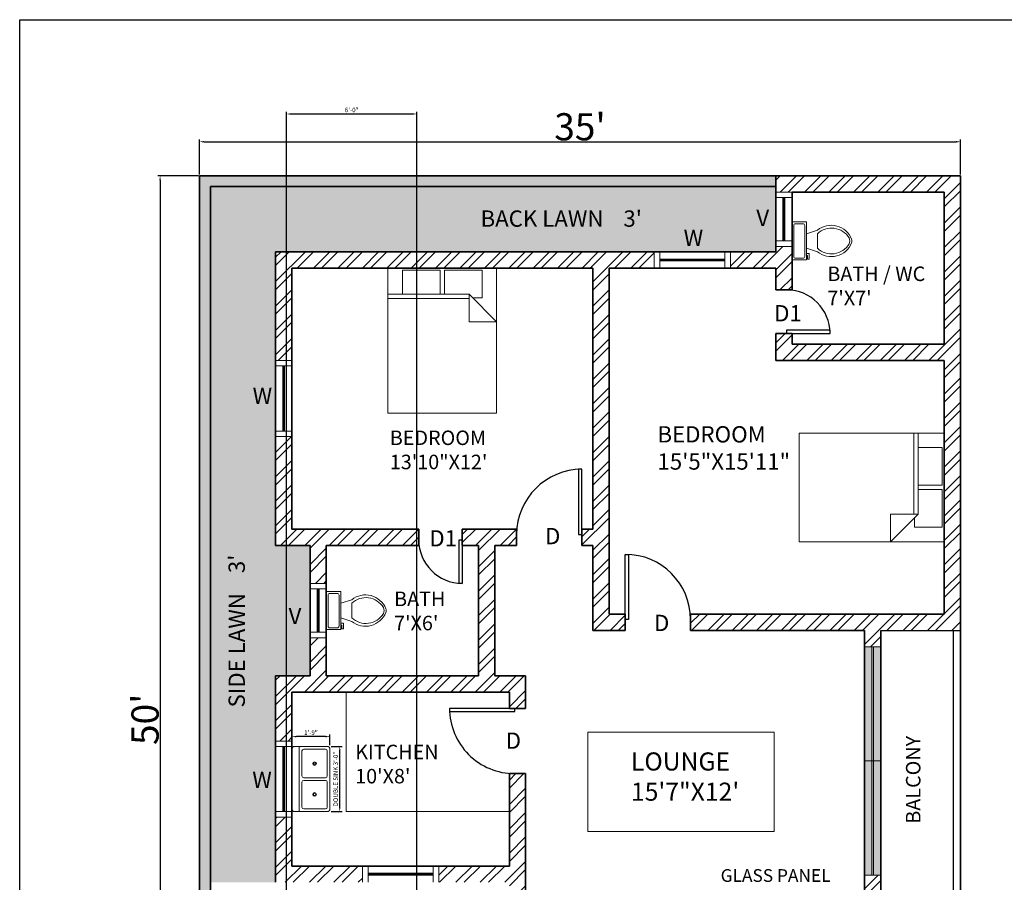
# Model space of a CAD drawing. Units: inches. Extents: x 2163 to 7246, y 928 to 2098.
# Tile 4 of 15: x 2163 to 2706, y 1622 to 2098. Entities that reach past the tile are written whole.
import ezdxf

# ---------------------------------------------------------------- set-up
doc = ezdxf.new("R2010")
doc.units = ezdxf.units.IN
for name, color, linetype, lineweight in [('A-ANNO-DIMS', 4, 'Continuous', 18), ('A-ANNO-TEXT', 7, 'Continuous', 18), ('A-ANNO-TTLB', 7, 'Continuous', 30), ('A-AREA-IDEN', 7, 'Continuous', 18), ('A-DOOR', 4, 'Continuous', 25), ('A-FLOR', 7, 'Continuous', 25), ('A-FLOR-FIXT', 9, 'Continuous', 20), ('A-FURN', 8, 'Continuous', 18), ('A-GLAZ', 30, 'Continuous', 20), ('A-WALL', 7, 'Continuous', 35), ('A-WALL-PATT', 8, 'Continuous', 13), ('C-PROP', 7, 'Continuous', 35), ('C-PROP-PATT', 4, 'Continuous', 13)]:
    doc.layers.add(name, color=color, linetype=linetype, lineweight=lineweight)
doc.layers.add('A-GLAZ-PATT', color=141, linetype='Continuous', lineweight=9, true_color=0xadddf7)
doc.layers.add('L-PLNT-PATT', color=85, linetype='Continuous', lineweight=13, true_color=0x58ba48)
doc.styles.get("Standard").update_dxf_attribs({"font": 'arial.ttf'})
doc.dimstyles.new('ISO-25', dxfattribs={"dimtxt": 2.5, "dimasz": 2.5, "dimexe": 1.25, "dimexo": 0.625, "dimtad": 1, "dimdec": 0, "dimlunit": 3, "dimtxsty": 'Standard', "dimcen": 2.5, "dimadec": 0, "dimazin": 0, "dimtfac": 1, "dimtdec": 0, "dimtmove": 0, "dimatfit": 3, "dimfxl": 1, "dimarcsym": 0})

# ---------------------------------------------------------------- blocks, each defined once
blk = doc.blocks.new('*U6')
for p, q in [((0, 0), (0, 6)), ((36, 0), (36, 6))]:
    blk.add_line(p, q)
blk.add_lwpolyline([(0, 0), (0, -36), (1.75, -36), (1.75, 0)], close=True)
blk.add_arc((0, 0), 36, 270, 0)
blk = doc.blocks.new('*U4')
for p, q in [((0, 0), (0, -6)), ((36, 0), (36, -6))]:
    blk.add_line(p, q)
blk.add_lwpolyline([(0, 0), (0, 36), (1.75, 36), (1.75, 0)], close=True)
blk.add_arc((0, 0), 36, 0, 90)
blk = doc.blocks.new('*U3')
for p, q in [((0, 0), (0, -6)), ((-36, 0), (-36, -6))]:
    blk.add_line(p, q)
blk.add_lwpolyline([(0, 0), (0, 36), (-1.75, 36), (-1.75, 0)], close=True)
blk.add_arc((0, 0), 36, 90, 180)
blk = doc.blocks.new('*U5')
for p, q in [((-24, 0), (-24, 6)), ((0, 0), (0, 6))]:
    blk.add_line(p, q)
blk.add_lwpolyline([(0, 0), (0, -24), (-1.75, -24), (-1.75, 0)], close=True)
blk.add_arc((0, 0), 24, 180, 270)
blk = doc.blocks.new('*U7')
for p, q in [((-24, 0), (-24, -6)), ((0, 0), (0, -6))]:
    blk.add_line(p, q)
blk.add_lwpolyline([(0, 0), (0, 24), (-1.75, 24), (-1.75, 0)], close=True)
blk.add_arc((0, 0), 24, 90, 180)
blk = doc.blocks.new('Bed - Queen')
for p, q in [((0, -80.00003), (0, 0)), ((0, 0), (59.99999, 0)), ((59.99999, 0), (59.99999, -80.00003)), ((7.99999, -1.2), (28.79998, -1.2)), ((7.99999, -14.4), (7.99999, -1.2)), ((28.79998, -1.2), (28.79998, -14.4)), ((31.19999, -1.2), (51.99999, -1.2)), ((31.19999, -14.4), (31.19999, -1.2)), ((51.99999, -1.2), (51.99999, -16.4)), ((0, -14.4), (44.8, -14.4)), ((59.99999, -29.6), (44.8, -14.4)), ((44.8, -14.4), (44.8, -29.6)), ((44.8, -16.8), (0, -16.8)), ((51.99999, -16.4), (46.79936, -16.4)), ((44.8, -29.6), (59.99999, -29.6)), ((59.99999, -80.00003), (0, -80.00003))]:
    blk.add_line(p, q)
blk = doc.blocks.new('Toilet - top')
for p, q in [((9.5, -6), (9.5, -2)), ((-10, -8.5), (-8, -8.5)), ((-10, -9.5), (-10, -8.5)), ((-7, -9.5), (-10, -9.5)), ((-8, -8.5), (-8, -8)), ((-7, -8), (-7, -9.5)), ((-4, -8), (-6, -14)), ((4, -8), (6, -14)), ((4, -14), (-4, -14))]:
    blk.add_line(p, q)
blk.add_lwpolyline([(10.5, -8), (10.5, 0), (-10.5, 0), (-10.5, -8)], close=True)
for points in [[(-9.5, -2), (-9.5, -6)], [(8.5, -1), (-8.5, -1)], [(-8.5, -7), (8.5, -7)]]:
    blk.add_lwpolyline(points)
for centre, radius, start, end in [((-8.62, -1.88), 0.884, 81.8699, 188.1301), ((8.62, -1.88), 0.884, 351.8699, 98.1301), ((-8.62, -6.12), 0.884, 171.8699, 278.1301), ((8.62, -6.12), 0.884, 261.8699, 8.1301), ((3.52, -21.58), 12.17, 141.4691, 247.9714), ((4.2, -21.82), 11.33, 136.3677, 238.9468), ((-3.52, -21.58), 12.17, 292.0284, 38.5307), ((-4.2, -21.82), 11.33, 301.053, 43.6321), ((0, -27.88), 4, 245.7318, 294.2682), ((0, -29), 4, 254.8605, 285.1395)]:
    blk.add_arc(centre, radius, start, end)
blk = doc.blocks.new('Sink-double - 36 in top')
for p, q in [((-18, -4), (18, -4)), ((-0.75, -18.5), (-0.75, -6.5)), ((0.75, -6.5), (0.75, -18.5))]:
    blk.add_line(p, q)
for points in [[(-16.5, 0), (16.5, 0)], [(-18, -19.5), (-18, -1.5)], [(18, -1.5), (18, -19.5)], [(-16.5, -18.5), (-16.5, -6.5)], [(-15.5, -5.5), (-1.75, -5.5)], [(1.75, -5.5), (15.5, -5.5)], [(16.5, -6.5), (16.5, -18.5)], [(16.5, -21), (-16.5, -21)], [(-1.75, -19.5), (-15.5, -19.5)], [(15.5, -19.5), (1.75, -19.5)]]:
    blk.add_lwpolyline(points)
for centre, radius in [((-8.5, -12.5), 1), ((-8.5, -12.5), 0.5), ((8.5, -12.5), 1), ((8.5, -12.5), 0.5)]:
    blk.add_circle(centre, radius)
for centre, radius, start, end in [((-16.5, -1.5), 1.5, 90, 180), ((16.5, -1.5), 1.5, 0, 90), ((-15.5, -6.5), 1, 90, 180), ((-1.75, -6.5), 1, 0, 90), ((1.75, -6.5), 1, 90, 180), ((15.5, -6.5), 1, 0, 90), ((-16.5, -19.5), 1.5, 180, 270), ((-15.5, -18.5), 1, 180, 270), ((-1.75, -18.5), 1, 270, 0), ((1.75, -18.5), 1, 180, 270), ((15.5, -18.5), 1, 270, 0), ((16.5, -19.5), 1.5, 270, 0)]:
    blk.add_arc(centre, radius, start, end)
blk = doc.blocks.new('*D19')
at = {"layer": 'A-ANNO-DIMS', "color": 0, "lineweight": -2, "transparency": 16777216}
for p, q in [((2261.84, 2012.7), (2261.84, 2032.07)), ((2264.34, 2030.82), (2679.34, 2030.82)), ((2681.84, 2012.7), (2681.84, 2032.07))]:
    blk.add_line(p, q, dxfattribs=at)
at = {"layer": 'A-ANNO-DIMS', "color": 0, "transparency": 16777216}
for points in [[(2264.34, 2031.24), (2264.34, 2030.41), (2261.84, 2030.82)], [(2679.34, 2031.24), (2679.34, 2030.41), (2681.84, 2030.82)]]:
    blk.add_solid(points, dxfattribs=at)
at = {"layer": 'Defpoints', "color": 0, "transparency": 16777216}
for p in [(2681.84, 2030.82), (2261.84, 2012.07), (2681.84, 2012.07)]:
    blk.add_point(p, dxfattribs=at)
at = {"layer": 'A-ANNO-DIMS', "color": 0, "transparency": 16777216, "insert": (2471.84, 2039.11), "char_height": 2.5, "attachment_point": 5}
blk.add_mtext("{\\H6x;35'}", dxfattribs=at)
blk = doc.blocks.new('*D20')
at = {"layer": 'A-ANNO-DIMS', "color": 0, "lineweight": -2, "transparency": 16777216}
for p, q in [((2261.22, 2012.07), (2238.85, 2012.07)), ((2240.1, 2009.57), (2240.1, 1414.57)), ((2261.22, 1412.07), (2238.85, 1412.07))]:
    blk.add_line(p, q, dxfattribs=at)
at = {"layer": 'A-ANNO-DIMS', "color": 0, "transparency": 16777216}
for points in [[(2239.68, 2009.57), (2240.52, 2009.57), (2240.1, 2012.07)], [(2239.68, 1414.57), (2240.52, 1414.57), (2240.1, 1412.07)]]:
    blk.add_solid(points, dxfattribs=at)
at = {"layer": 'Defpoints', "color": 0, "transparency": 16777216}
for p in [(2261.84, 2012.07), (2240.1, 1412.07), (2261.84, 1412.07)]:
    blk.add_point(p, dxfattribs=at)
at = {"layer": 'A-ANNO-DIMS', "color": 0, "transparency": 16777216, "insert": (2231.81, 1712.07), "char_height": 2.5, "attachment_point": 5, "rotation": 90}
blk.add_mtext("{\\H6x;50'}", dxfattribs=at)
blk = doc.blocks.new('WIN-36-PLAN')
for p, q in [((0, 9), (0, 0)), ((3, 9), (3, 0)), ((39, 9), (39, 0)), ((42, 9), (42, 0)), ((3, 5), (39, 5)), ((3, 4.5), (39, 4.5)), ((3, 4), (39, 4))]:
    blk.add_line(p, q)
blk = doc.blocks.new('VENT-24-PLAN')
for p, q in [((9, 30), (0, 30)), ((9, 27), (0, 27)), ((4, 27), (4, 3)), ((4.5, 27), (4.5, 3)), ((5, 27), (5, 3)), ((9, 3), (0, 3)), ((9, 0), (0, 0))]:
    blk.add_line(p, q)
blk = doc.blocks.new('*D73')
at = {"layer": 'A-ANNO-DIMS', "color": 0, "lineweight": -2, "transparency": 16777216}
for p, q in [((2334.47, 1697.07), (2340.49, 1697.07)), ((2339.24, 1663.57), (2339.24, 1694.57)), ((2334.47, 1661.07), (2340.49, 1661.07))]:
    blk.add_line(p, q, dxfattribs=at)
at = {"layer": 'A-ANNO-DIMS', "color": 0, "transparency": 16777216}
for points in [[(2338.83, 1694.57), (2339.66, 1694.57), (2339.24, 1697.07)], [(2338.83, 1663.57), (2339.66, 1663.57), (2339.24, 1661.07)]]:
    blk.add_solid(points, dxfattribs=at)
at = {"layer": 'Defpoints', "color": 0, "transparency": 16777216}
for p in [(2333.84, 1697.07), (2339.24, 1697.07), (2333.84, 1661.07)]:
    blk.add_point(p, dxfattribs=at)
at = {"layer": 'A-ANNO-DIMS', "color": 0, "transparency": 16777216, "insert": (2337.32, 1679.07), "char_height": 2.5, "attachment_point": 5, "rotation": 90}
blk.add_mtext('DOUBLE SINK 3\'-0"', dxfattribs=at)
blk = doc.blocks.new('*D74')
at = {"layer": 'A-ANNO-DIMS', "color": 0, "lineweight": -2, "transparency": 16777216}
for p, q in [((2312.84, 1697.7), (2312.84, 1703.72)), ((2331.34, 1702.47), (2315.34, 1702.47)), ((2333.84, 1697.7), (2333.84, 1703.72))]:
    blk.add_line(p, q, dxfattribs=at)
at = {"layer": 'A-ANNO-DIMS', "color": 0, "transparency": 16777216}
for points in [[(2315.34, 1702.89), (2315.34, 1702.06), (2312.84, 1702.47)], [(2331.34, 1702.89), (2331.34, 1702.06), (2333.84, 1702.47)]]:
    blk.add_solid(points, dxfattribs=at)
at = {"layer": 'Defpoints', "color": 0, "transparency": 16777216}
for p in [(2312.84, 1702.47), (2312.84, 1697.07), (2333.84, 1697.07)]:
    blk.add_point(p, dxfattribs=at)
at = {"layer": 'A-ANNO-DIMS', "color": 0, "transparency": 16777216, "insert": (2323.34, 1704.37), "char_height": 2.5, "attachment_point": 5}
blk.add_mtext('1\'-9"', dxfattribs=at)
blk = doc.blocks.new('*D78')
at = {"layer": 'A-ANNO-DIMS', "color": 0, "lineweight": -2, "transparency": 16777216}
for p, q in [((2309.84, 1412.7), (2309.84, 2047.42)), ((2312.34, 2046.17), (2379.34, 2046.17)), ((2381.84, 1412.7), (2381.84, 2047.42))]:
    blk.add_line(p, q, dxfattribs=at)
at = {"layer": 'A-ANNO-DIMS', "color": 0, "transparency": 16777216}
for points in [[(2312.34, 2046.59), (2312.34, 2045.76), (2309.84, 2046.17)], [(2379.34, 2046.59), (2379.34, 2045.76), (2381.84, 2046.17)]]:
    blk.add_solid(points, dxfattribs=at)
at = {"layer": 'Defpoints', "color": 0, "transparency": 16777216}
for p in [(2381.84, 2046.17), (2309.84, 1412.07), (2381.84, 1412.07)]:
    blk.add_point(p, dxfattribs=at)
at = {"layer": 'A-ANNO-DIMS', "color": 0, "transparency": 16777216, "insert": (2345.84, 2048.07), "char_height": 2.5, "attachment_point": 5}
blk.add_mtext('6\'-0"', dxfattribs=at)

msp = doc.modelspace()

# ---------------------------------------------------------------- hatches: boundary and pattern name
at = {"layer": 'A-GLAZ-PATT'}
h = msp.add_hatch(color=256, dxfattribs=at)
h.dxf.hatch_style = 1
h.paths.add_polyline_path([(2632.84, 1689.07), (2628.84, 1689.07), (2628.84, 1626.07), (2632.84, 1626.07)])
h.paths.add_polyline_path([(2637.84, 1689.07), (2633.84, 1689.07), (2633.84, 1626.07), (2637.84, 1626.07)])
h.paths.add_polyline_path([(2633.84, 1689.07), (2632.84, 1689.07), (2632.84, 1626.07), (2633.84, 1626.07)])
h.paths.add_polyline_path([(2637.84, 1752.07), (2633.84, 1752.07), (2633.84, 1689.07), (2637.84, 1689.07)])
h.paths.add_polyline_path([(2632.84, 1752.07), (2628.84, 1752.07), (2628.84, 1689.07), (2632.84, 1689.07)])
h.paths.add_polyline_path([(2633.84, 1752.07), (2632.84, 1752.07), (2632.84, 1689.07), (2633.84, 1689.07)])
at = {"layer": 'A-WALL-PATT'}
h = msp.add_hatch(dxfattribs=at)
h.set_pattern_fill('ANSI32', color=256)
h.paths.add_polyline_path([(2637.84, 1761.07), (2681.84, 1761.07), (2681.84, 2012.07), (2579.84, 2012.07), (2579.84, 2003.07), (2588.84, 2003.07), (2672.84, 2003.07), (2672.84, 1919.07), (2588.84, 1919.07), (2588.84, 1925.07), (2579.84, 1925.07), (2579.84, 1910.07), (2672.84, 1910.07), (2672.84, 1770.07), (2532.84, 1770.07), (2532.84, 1761.07), (2628.84, 1761.07), (2628.84, 1752.07), (2637.84, 1752.07)])
h.paths.add_polyline_path([(2496.84, 1761.07), (2496.84, 1770.07), (2487.84, 1770.07), (2487.84, 1961.07), (2512.84, 1961.07), (2512.84, 1970.07), (2303.84, 1970.07), (2303.84, 1910.07), (2312.84, 1910.07), (2312.84, 1961.07), (2478.84, 1961.07), (2478.84, 1817.07), (2472.84, 1817.07), (2472.84, 1808.07), (2478.84, 1808.07), (2478.84, 1761.07)])
h.paths.add_polyline_path([(2331.84, 1808.07), (2337.84, 1808.07), (2382.84, 1808.07), (2382.84, 1817.07), (2337.84, 1817.07), (2312.84, 1817.07), (2312.84, 1868.07), (2303.84, 1868.07), (2303.84, 1808.07), (2322.84, 1808.07), (2322.84, 1787.07), (2331.84, 1787.07)], flags=17)
h.paths.add_polyline_path([(2579.84, 1961.07), (2579.84, 1949.07), (2585.84, 1949.07), (2588.84, 1949.07), (2588.84, 1973.07), (2579.84, 1973.07), (2579.84, 1970.07), (2554.84, 1970.07), (2554.84, 1961.07)], flags=17)
h = msp.add_hatch(dxfattribs=at)
h.set_pattern_fill('ANSI32', color=256)
h.paths.add_polyline_path([(2461.84, 1464.07), (2441.84, 1464.07), (2441.84, 1562.07), (2432.84, 1562.07), (2432.84, 1455.07), (2461.84, 1455.07)])
h.paths.add_polyline_path([(2575.84, 1464.07), (2532.84, 1464.07), (2532.84, 1548.07), (2523.84, 1548.07), (2523.84, 1464.07), (2503.84, 1464.07), (2503.84, 1455.07), (2575.84, 1455.07)])
h.paths.add_polyline_path([(2681.84, 1617.07), (2637.84, 1617.07), (2637.84, 1626.07), (2628.84, 1626.07), (2628.84, 1617.07), (2616.84, 1617.07), (2616.84, 1608.07), (2672.84, 1608.07), (2672.84, 1464.07), (2629.84, 1464.07), (2629.84, 1455.07), (2672.84, 1455.07), (2672.84, 1412.07), (2681.84, 1412.07)])
h.paths.add_polyline_path([(2544.84, 1617.07), (2523.84, 1617.07), (2523.84, 1596.07), (2532.84, 1596.07), (2532.84, 1608.07), (2544.84, 1608.07)])
h.paths.add_polyline_path([(2441.84, 1682.07), (2432.84, 1682.07), (2432.84, 1631.07), (2393.84, 1631.07), (2393.84, 1622.07), (2432.84, 1622.07), (2432.84, 1610.07), (2441.84, 1610.07)])
h.paths.add_polyline_path([(2441.84, 1736.07), (2424.84, 1736.07), (2424.84, 1808.07), (2436.84, 1808.07), (2436.84, 1817.07), (2406.84, 1817.07), (2406.84, 1808.07), (2415.84, 1808.07), (2415.84, 1736.07), (2331.84, 1736.07), (2331.84, 1757.07), (2322.84, 1757.07), (2322.84, 1736.07), (2303.84, 1736.07), (2303.84, 1700.07), (2312.84, 1700.07), (2312.84, 1727.07), (2432.84, 1727.07), (2432.84, 1718.07), (2441.84, 1718.07)])
h.paths.add_polyline_path([(2351.84, 1631.07), (2312.84, 1631.07), (2312.84, 1658.07), (2303.84, 1658.07), (2303.84, 1622.07), (2351.84, 1622.07)])
at = {"layer": 'C-PROP-PATT'}
h = msp.add_hatch(dxfattribs=at)
h.set_pattern_fill('ANSI35', color=256)
h.paths.add_polyline_path([(2309.84, 1418.07), (2267.84, 1418.07), (2267.84, 2006.07), (2579.84, 2006.07), (2579.84, 2012.07), (2261.84, 2012.07), (2261.84, 1412.07), (2309.84, 1412.07)])
at = {"layer": 'L-PLNT-PATT'}
h = msp.add_hatch(dxfattribs=at)
h.set_pattern_fill('CROSS', color=256)
h.paths.add_polyline_path([(2579.84, 2006.07), (2267.84, 2006.07), (2267.84, 1622.07), (2303.84, 1622.07), (2303.84, 1736.07), (2322.84, 1736.07), (2322.84, 1808.07), (2303.84, 1808.07), (2303.84, 1970.07), (2579.84, 1970.07)])
h.paths.add_polyline_path([(2672.84, 1455.07), (2432.84, 1455.07), (2432.84, 1418.07), (2672.84, 1418.07)])
h.paths.add_polyline_path([(2291.95, 1715.76), (2291.95, 1812.79), (2273.41, 1812.79), (2273.41, 1715.76)], flags=24)
h.paths.add_polyline_path([(2413.78, 1978.86), (2515.7, 1978.86), (2515.7, 1997.41), (2413.78, 1997.41)], flags=24)
h.paths.add_polyline_path([(2509.67, 1423.19), (2632.98, 1423.19), (2632.98, 1443.8), (2509.67, 1443.8)], flags=24)

# ---------------------------------------------------------------- linework, layer by layer
at = {"layer": 'A-ANNO-TTLB'}
msp.add_lwpolyline([(2162.62, 2098.21), (3633.38, 2098.21), (3633.38, 928.48), (2162.62, 928.48)], close=True, dxfattribs=at)
at = {"layer": 'A-AREA-IDEN'}
msp.add_lwpolyline([(2476.13, 1704.87), (2579.05, 1704.87), (2579.05, 1650.15), (2476.13, 1650.15)], close=True, dxfattribs=at)
at = {"layer": 'A-FLOR'}
for p, q in [((2637.84, 1761.07), (2681.84, 1761.07)), ((2677.84, 1761.07), (2677.84, 1617.07))]:
    msp.add_line(p, q, dxfattribs=at)
at = {"layer": 'A-FLOR-FIXT'}
for q in [(2342.84, 1727.07), (2432.84, 1661.07)]:
    msp.add_line((2342.84, 1661.07), q, dxfattribs=at)
at = {"layer": 'A-GLAZ'}
for p, q in [((2628.84, 1752.07), (2637.84, 1752.07)), ((2632.84, 1752.07), (2632.84, 1626.07)), ((2633.84, 1752.07), (2633.84, 1626.07)), ((2628.84, 1689.07), (2637.84, 1689.07)), ((2628.84, 1626.07), (2637.84, 1626.07))]:
    msp.add_line(p, q, dxfattribs=at)
at = {"layer": 'A-WALL'}
for p, q in [((2579.84, 2012.07), (2579.84, 1970.07)), ((2588.84, 2003.07), (2588.84, 1949.07)), ((2588.84, 2003.07), (2672.84, 2003.07)), ((2672.84, 2003.07), (2672.84, 1919.07)), ((2303.84, 1808.07), (2303.84, 1970.07)), ((2303.84, 1970.07), (2579.84, 1970.07)), ((2312.84, 1817.07), (2312.84, 1961.07)), ((2312.84, 1961.07), (2478.84, 1961.07)), ((2478.84, 1961.07), (2478.84, 1817.07)), ((2487.84, 1961.07), (2487.84, 1770.07)), ((2487.84, 1961.07), (2579.84, 1961.07)), ((2579.84, 1961.07), (2579.84, 1949.07)), ((2579.84, 1949.07), (2588.84, 1949.07)), ((2579.84, 1925.07), (2588.84, 1925.07)), ((2579.84, 1925.07), (2579.84, 1910.07)), ((2588.84, 1925.07), (2588.84, 1919.07)), ((2588.84, 1919.07), (2672.84, 1919.07)), ((2579.84, 1910.07), (2672.84, 1910.07)), ((2672.84, 1910.07), (2672.84, 1770.07)), ((2312.84, 1817.07), (2337.84, 1817.07)), ((2337.84, 1817.07), (2382.84, 1817.07)), ((2382.84, 1817.07), (2382.84, 1808.07)), ((2406.84, 1817.07), (2406.84, 1808.07)), ((2406.84, 1817.07), (2436.84, 1817.07)), ((2436.84, 1817.07), (2436.84, 1808.07)), ((2472.84, 1817.07), (2472.84, 1808.07)), ((2472.84, 1817.07), (2478.84, 1817.07)), ((2303.84, 1808.07), (2322.84, 1808.07)), ((2322.84, 1808.07), (2322.84, 1736.07)), ((2331.84, 1808.07), (2331.84, 1736.07)), ((2331.84, 1808.07), (2337.84, 1808.07)), ((2337.84, 1808.07), (2382.84, 1808.07)), ((2406.84, 1808.07), (2415.84, 1808.07)), ((2415.84, 1808.07), (2415.84, 1736.07)), ((2424.84, 1808.07), (2424.84, 1736.07)), ((2424.84, 1808.07), (2436.84, 1808.07)), ((2472.84, 1808.07), (2478.84, 1808.07)), ((2478.84, 1808.07), (2478.84, 1761.07)), ((2487.84, 1770.07), (2496.84, 1770.07)), ((2496.84, 1770.07), (2496.84, 1761.07)), ((2532.84, 1770.07), (2532.84, 1761.07)), ((2532.84, 1770.07), (2672.84, 1770.07)), ((2478.84, 1761.07), (2496.84, 1761.07)), ((2532.84, 1761.07), (2628.84, 1761.07)), ((2628.84, 1617.07), (2628.84, 1761.07)), ((2637.84, 1617.07), (2637.84, 1761.07)), ((2303.84, 1622.07), (2303.84, 1736.07)), ((2303.84, 1736.07), (2322.84, 1736.07)), ((2331.84, 1736.07), (2415.84, 1736.07)), ((2424.84, 1736.07), (2441.84, 1736.07)), ((2441.84, 1718.07), (2441.84, 1736.07)), ((2312.84, 1631.07), (2312.84, 1727.07)), ((2312.84, 1727.07), (2432.84, 1727.07)), ((2432.84, 1718.07), (2432.84, 1727.07)), ((2432.84, 1718.07), (2441.84, 1718.07)), ((2432.84, 1631.07), (2432.84, 1682.07)), ((2432.84, 1682.07), (2441.84, 1682.07)), ((2441.84, 1610.07), (2441.84, 1682.07)), ((2312.84, 1631.07), (2432.84, 1631.07))]:
    msp.add_line(p, q, dxfattribs=at)
at = {"layer": 'C-PROP'}
for p, q in [((2261.84, 2012.07), (2681.84, 2012.07)), ((2261.84, 1412.07), (2261.84, 2012.07)), ((2681.84, 2012.07), (2681.84, 1412.07)), ((2267.84, 2006.07), (2579.84, 2006.07)), ((2267.84, 1418.07), (2267.84, 2006.07))]:
    msp.add_line(p, q, dxfattribs=at)

# ---------------------------------------------------------------- block references
at = {"layer": 'A-DOOR', "rotation": 270}
for name, p in [('*U7', (2585.84, 1925.07)), ('*U6', (2435.84, 1718.07))]:
    msp.add_blockref(name, p, dxfattribs=at)
at = {"layer": 'A-DOOR'}
for name, p in [('*U3', (2472.84, 1814.07)), ('*U5', (2406.84, 1811.07)), ('*U4', (2496.84, 1767.07))]:
    msp.add_blockref(name, p, dxfattribs=at)
at = {"layer": 'A-FLOR-FIXT', "rotation": 90}
for name, p in [('Toilet - top', (2588.84, 1976.07)), ('Toilet - top', (2331.84, 1772.07)), ('Sink-double - 36 in top', (2312.84, 1679.07))]:
    msp.add_blockref(name, p, dxfattribs=at)
at = {"layer": 'A-FURN'}
msp.add_blockref('Bed - Queen', (2365.84, 1961.07), dxfattribs=at)
at = {"layer": 'A-FURN', "rotation": 270}
msp.add_blockref('Bed - Queen', (2672.84, 1870.07), dxfattribs=at)
at = {"layer": 'A-GLAZ'}
for name, p in [('VENT-24-PLAN', (2579.84, 1973.07)), ('WIN-36-PLAN', (2512.84, 1961.07)), ('VENT-24-PLAN', (2322.84, 1757.07)), ('WIN-36-PLAN', (2351.84, 1622.07))]:
    msp.add_blockref(name, p, dxfattribs=at)
at = {"layer": 'A-GLAZ', "rotation": 90}
for p in [(2312.84, 1868.07), (2312.84, 1658.07)]:
    msp.add_blockref('WIN-36-PLAN', p, dxfattribs=at)

# ---------------------------------------------------------------- texts
at = {"layer": 'A-ANNO-TEXT', "attachment_point": 1}
for s, insert, char_height in [('V', (2569.14, 1993.3), 9), ('W', (2529.04, 1982.27), 9), ('D1', (2579, 1940.66), 9), ('W', (2291.17, 1895.14), 9), ('D1', (2388.69, 1816.44), 9), ('D', (2452.54, 1817.67), 9), ('V', (2311.01, 1773.56), 9), ('D', (2512.67, 1769.74), 9), ('D', (2430.85, 1704.76), 9), ('W', (2290.97, 1683.22), 9), ('GLASS PANEL', (2549.45, 1629.33), 7)]:
    msp.add_mtext_dynamic_manual_height_columns(s, width=361.5259, gutter_width=12.5, heights=[0], dxfattribs=dict(at, insert=insert, char_height=char_height))
at = {"layer": 'A-AREA-IDEN', "attachment_point": 1}
for s, width, insert, char_height in [("BACK LAWN    3'", 398.0544, (2416.95, 1992.93), 9), ("BATH / WC\\P7'X7'", 344.4804, (2608.35, 1961.95), 8), ('BEDROOM\\P13\'10"X12\'', 462.4335, (2366.88, 1871.43), 8), ('BEDROOM\\P15\'5"X15\'11"', 720.8452, (2514.59, 1873.84), 9), ("BATH \\P7'X6'", 208.9594, (2369.25, 1782.53), 8), ("KITCHEN\\P10'X8'", 70.9924, (2347.76, 1698.01), 8), ('LOUNGE\\P15\'7"X12\'', 90.7352, (2499.96, 1693.77), 10)]:
    msp.add_mtext_dynamic_manual_height_columns(s, width=width, gutter_width=12.5, heights=[0], dxfattribs=dict(at, insert=insert, char_height=char_height))
at = {"layer": 'A-AREA-IDEN', "attachment_point": 1, "rotation": 90}
for s, width, insert, char_height in [("SIDE LAWN    3' ", 526.893, (2277.89, 1718.58), 9), ('BALCONY', 218.1461, (2651.72, 1654.42), 8)]:
    msp.add_mtext_dynamic_manual_height_columns(s, width=width, gutter_width=12.5, heights=[0], dxfattribs=dict(at, insert=insert, char_height=char_height))

# ---------------------------------------------------------------- dimensions: what is measured, and where the dimension line sits
at = {"layer": 'A-ANNO-DIMS'}
dim = msp.add_linear_dim(base=(2381.84, 2046.17), p1=(2309.84, 1412.07), p2=(2381.84, 1412.07), dimstyle='ISO-25', override={"dimdec": 1, "dimlfac": 1, "dimrnd": 0, "dimzin": 1, "dimdsep": 46, "dimlunit": 4, "dimfrac": 2}, dxfattribs=at)
dim.commit()
dim.dimension.update_dxf_attribs({"geometry": '*D78', "text_midpoint": (2345.84, 2048.07)})
dim = msp.add_linear_dim(base=(2681.84, 2030.82), p1=(2261.84, 2012.07), p2=(2681.84, 2012.07), text='{\\H6x;<>}', dimstyle='ISO-25', override={"dimclrd": 0, "dimclre": 0, "dimclrt": 0}, dxfattribs=at)
dim.commit()
dim.dimension.update_dxf_attribs({"geometry": '*D19', "text_midpoint": (2471.84, 2030.82), "dimtype": 160})
for base, p1, p2, text, override, picture, middle in [((2240.1, 1412.07), (2261.84, 2012.07), (2261.84, 1412.07), '{\\H6x;<>}', {"dimclrd": 0, "dimclre": 0, "dimclrt": 0}, '*D20', (2231.81, 1712.07)), ((2339.24, 1697.07), (2333.84, 1661.07), (2333.84, 1697.07), 'DOUBLE SINK <>', {"dimdec": 1, "dimlfac": 1, "dimrnd": 0, "dimzin": 1, "dimdsep": 46, "dimlunit": 4, "dimfrac": 2}, '*D73', (2337.32, 1679.07))]:
    dim = msp.add_linear_dim(base=base, p1=p1, p2=p2, angle=90, text=text, dimstyle='ISO-25', override=override, dxfattribs=at)
    dim.commit()
    dim.dimension.update_dxf_attribs({"geometry": picture, "text_midpoint": middle})
dim = msp.add_linear_dim(base=(2312.84, 1702.47), p1=(2333.84, 1697.07), p2=(2312.84, 1697.07), angle=180, dimstyle='ISO-25', override={"dimdec": 1, "dimlfac": 1, "dimrnd": 0, "dimzin": 1, "dimdsep": 46, "dimlunit": 4, "dimfrac": 2}, dxfattribs=at)
dim.commit()
dim.dimension.update_dxf_attribs({"geometry": '*D74', "text_midpoint": (2323.34, 1704.37)})

doc.saveas('drawing.dxf')
